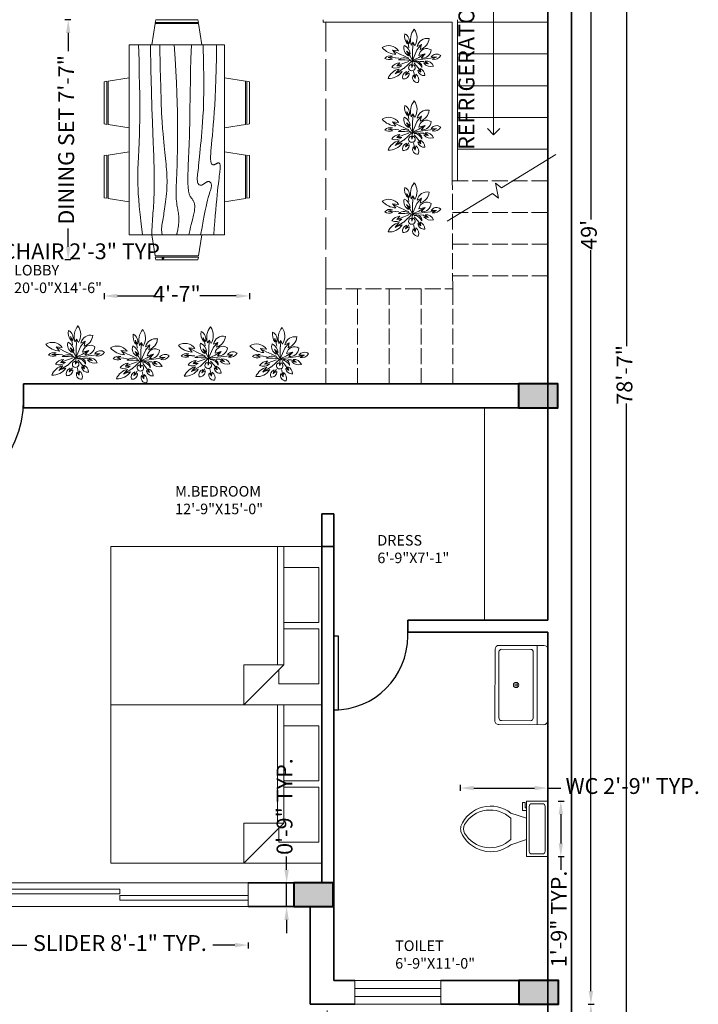
# Model space of a CAD drawing. Units: inches. Extents: x 2845 to 3575, y 808 to 1996.
# Tile 4 of 6: x 3304 to 3561, y 1215 to 1588. Entities that reach past the tile are written whole.
import ezdxf

# ---------------------------------------------------------------- set-up
doc = ezdxf.new("R2010")
doc.units = ezdxf.units.IN
doc.linetypes.add('ACAD_ISO02W100', pattern=[15, 12, -3])
for name, color, linetype, lineweight in [('A-ANNO-DIMS', 2, 'Continuous', 18), ('A-ANNO-SYMB', 7, 'Continuous', 18), ('A-AREA-IDEN', 7, 'Continuous', 18), ('A-COLS', 7, 'Continuous', 40), ('A-DOOR', 34, 'Continuous', 25), ('A-FLOR-CASE', 30, 'Continuous', 18), ('A-FLOR-FIXT', 8, 'Continuous', 18), ('A-FLOR-STRS', 142, 'Continuous', 18), ('A-FLOR-STRS-OVHD', 142, 'ACAD_ISO02W100', 18), ('A-FURN', 30, 'Continuous', 18), ('A-GLAZ', 4, 'Continuous', 18), ('A-ROOF-OVHD', 7, 'ACAD_ISO02W100', 18), ('A-WALL', 1, 'Continuous', 35), ('L-PLNT', 3, 'Continuous', 13)]:
    doc.layers.add(name, color=color, linetype=linetype, lineweight=lineweight)
doc.styles.get("Standard").update_dxf_attribs({"font": 'arial.ttf'})
doc.dimstyles.new('ISO-25', dxfattribs={"dimtxt": 6, "dimasz": 5, "dimexe": 1.25, "dimexo": 0.625, "dimtad": 0, "dimlunit": 4, "dimtxsty": 'Standard', "dimcen": 2.5, "dimclrd": 1, "dimclre": 1, "dimclrt": 1, "dimadec": 0, "dimazin": 0, "dimtfac": 1, "dimtmove": 0, "dimatfit": 3, "dimfxl": 1, "dimfxlon": 1, "dimfrac": 1, "dimarcsym": 0})

# ---------------------------------------------------------------- blocks, each defined once
blk = doc.blocks.new('*U5')
for p, q in [((0, 0), (0, 6)), ((40, 0), (40, 6))]:
    blk.add_line(p, q)
blk.add_lwpolyline([(0, 0), (0, -40), (1.75, -40), (1.75, 0)], close=True)
blk.add_arc((0, 0), 40, 270, 0)
blk = doc.blocks.new('*U6')
for p, q in [((0, 0), (0, 6)), ((28, 0), (28, 6))]:
    blk.add_line(p, q)
blk.add_lwpolyline([(0, 0), (0, -28), (1.75, -28), (1.75, 0)], close=True)
blk.add_arc((0, 0), 28, 270, 0)
blk = doc.blocks.new('Bed - Queen')
for p, q in [((0, -80.00003), (0, 0)), ((0, 0), (59.99999, 0)), ((59.99999, 0), (59.99999, -80.00003)), ((7.99999, -1.2), (28.79998, -1.2)), ((7.99999, -14.4), (7.99999, -1.2)), ((28.79998, -1.2), (28.79998, -14.4)), ((31.19999, -1.2), (51.99999, -1.2)), ((31.19999, -14.4), (31.19999, -1.2)), ((51.99999, -1.2), (51.99999, -16.4)), ((0, -14.4), (44.8, -14.4)), ((59.99999, -29.6), (44.8, -14.4)), ((44.8, -14.4), (44.8, -29.6)), ((44.8, -16.8), (0, -16.8)), ((51.99999, -16.4), (46.79936, -16.4)), ((44.8, -29.6), (59.99999, -29.6)), ((59.99999, -80.00003), (0, -80.00003))]:
    blk.add_line(p, q)
blk = doc.blocks.new('Dining Set - 36 x 72 in.')
for p, q in [((-22, 27.5), (-22.1562, 26.50042)), ((-5.8416, 26.5), (-22.1534, 26.5)), ((-22, 27.5), (-6, 27.5)), ((-5.8437, 26.49966), (-6, 27.5)), ((6, 27.5), (5.8438, 26.50042)), ((22.1584, 26.5), (5.8466, 26.5)), ((6, 27.5), (22, 27.5)), ((22.1563, 26.49966), (22, 27.5)), ((-22.2343, 26.00059), (-23.4847, 17.99762)), ((-22.2304, 26), (-5.7608, 26)), ((-4.5152, 17.99762), (-5.7655, 25.99926)), ((5.7657, 26.00059), (4.5153, 17.99762)), ((5.7696, 26), (22.2392, 26)), ((23.4848, 17.99762), (22.2345, 25.99926)), ((36, 18), (-36, 18)), ((-36, 18), (-36, -18)), ((36, -18), (36, 18)), ((-45.5, 8), (-44.5004, 8.15617)), ((-45.5, 8), (-45.5, -8)), ((-44.5, -8.15843), (-44.5, 8.15338)), ((-44.0006, 8.23428), (-35.9976, 9.48474)), ((-44, 8.23041), (-44, -8.23915)), ((44.0006, 8.23428), (35.9976, 9.48474)), ((44, 8.23041), (44, -8.23915)), ((44.5, -8.15843), (44.5, 8.15338)), ((45.5, 8), (44.5005, 8.15617)), ((45.5, 8), (45.5, -8)), ((-44.4997, -8.15631), (-45.5, -8)), ((-35.9976, -9.48476), (-43.9993, -8.2345)), ((35.9976, -9.48476), (43.9993, -8.2345)), ((44.4997, -8.15631), (45.5, -8)), ((-36, -18), (36, -18)), ((-22.2343, -26.0006), (-23.4847, -17.99762)), ((-4.5152, -17.99762), (-5.7655, -25.99928)), ((5.7657, -26.0006), (4.5153, -17.99762)), ((23.4848, -17.99762), (22.2345, -25.99928)), ((-22.2304, -26), (-5.7608, -26)), ((5.7696, -26), (22.2392, -26)), ((-22, -27.5), (-22.1562, -26.50044)), ((-5.8416, -26.5), (-22.1534, -26.5)), ((-22, -27.5), (-6, -27.5)), ((-5.8437, -26.49967), (-6, -27.5)), ((6, -27.5), (5.8438, -26.50044)), ((22.1584, -26.5), (5.8466, -26.5)), ((6, -27.5), (22, -27.5)), ((22.1563, -26.49967), (22, -27.5))]:
    blk.add_line(p, q)
for points in [[(-36, 15), (-31.1772, 14.97754), (-26.8079, 14.91406), (-22.8538, 14.81543), (-19.276, 14.6875), (-16.0362, 14.53613), (-13.0957, 14.36718), (-10.4159, 14.18652), (-7.9583, 14), (-5.6904, 13.81315), (-3.6035, 13.63021), (-1.6954, 13.45508), (0.0365, 13.29166), (1.5945, 13.14388), (2.9811, 13.01562), (4.1988, 12.9108), (5.25, 12.83333), (6.1393, 12.78613), (6.8802, 12.76823), (7.4883, 12.77767), (7.9792, 12.8125), (8.3685, 12.87077), (8.6719, 12.95052), (8.9049, 13.0498), (9.0833, 13.16666), (9.2205, 13.29899), (9.3216, 13.44401), (9.3895, 13.59879), (9.4271, 13.76041), (9.4373, 13.92594), (9.4232, 14.09245), (9.3875, 14.257), (9.3333, 14.41666), (9.2638, 14.56917), (9.1836, 14.71484), (9.0975, 14.85465), (9.0104, 14.98958), (8.9272, 15.1206), (8.8529, 15.2487), (8.7922, 15.37483), (8.75, 15.5), (8.7305, 15.62467), (8.7344, 15.74739), (8.7617, 15.86621), (8.8125, 15.97916), (8.8867, 16.08431), (8.9844, 16.17968), (9.1055, 16.26334), (9.25, 16.33333), (9.4189, 16.38802), (9.6172, 16.42708), (9.8506, 16.45052), (10.125, 16.45833), (10.4463, 16.45052), (10.8203, 16.42708), (11.2529, 16.38802), (11.75, 16.33333), (12.3184, 16.26318), (12.9694, 16.17838), (13.7151, 16.07991), (14.5677, 15.96875), (15.5395, 15.84586), (16.6426, 15.71224), (17.8893, 15.56884), (19.2917, 15.41666), (20.859, 15.25667), (22.5879, 15.08984), (24.4721, 14.91715), (26.5052, 14.73958), (28.6809, 14.5581), (30.9929, 14.3737), (33.4347, 14.18733), (36, 14)], [(-36, 10), (-28.9766, 10.14274), (-23.1725, 10.20442), (-18.4241, 10.19775), (-14.5677, 10.13541), (-11.4399, 10.03011), (-8.877, 9.89453), (-6.7154, 9.74137), (-4.7917, 9.58333), (-2.9698, 9.43082), (-1.2246, 9.28515), (0.4415, 9.14534), (2.026, 9.01041), (3.5266, 8.87939), (4.9408, 8.7513), (6.266, 8.62516), (7.5, 8.5), (8.6411, 8.37549), (9.6914, 8.2539), (10.6538, 8.13818), (11.5312, 8.03125), (12.3267, 7.93603), (13.043, 7.85547), (13.6831, 7.79248), (14.25, 7.75), (14.7471, 7.7303), (15.1797, 7.73307), (15.5537, 7.75732), (15.875, 7.80208), (16.1494, 7.86637), (16.3828, 7.94922), (16.5811, 8.04964), (16.75, 8.16666), (16.8944, 8.29915), (17.0143, 8.44531), (17.1089, 8.60319), (17.1771, 8.77083), (17.218, 8.94629), (17.2305, 9.1276), (17.2137, 9.31282), (17.1667, 9.5), (17.0895, 9.6875), (16.987, 9.875), (16.8649, 10.0625), (16.7292, 10.25), (16.5856, 10.4375), (16.4401, 10.625), (16.2985, 10.8125), (16.1667, 11), (16.05, 11.18733), (15.9518, 11.3737), (15.8752, 11.5581), (15.8229, 11.73958), (15.798, 11.91715), (15.8034, 12.08984), (15.842, 12.25667), (15.9167, 12.41666), (16.0295, 12.56836), (16.1784, 12.70833), (16.3605, 12.83268), (16.5729, 12.9375), (16.8127, 13.01888), (17.0768, 13.07291), (17.3625, 13.0957), (17.6667, 13.08333), (17.9894, 13.03312), (18.3418, 12.94726), (18.7382, 12.82918), (19.1927, 12.68229), (19.7195, 12.51001), (20.3327, 12.31575), (21.0465, 12.10294), (21.875, 11.875), (22.8357, 11.63354), (23.959, 11.37304), (25.2786, 11.08618), (26.8282, 10.76562), (28.6414, 10.40405), (30.752, 9.99414), (33.1936, 9.52856), (36, 9)], [(-36, 5.5), (-30.7157, 5.3348), (-26.069, 5.20963), (-21.9946, 5.11767), (-18.4271, 5.05208), (-15.3009, 5.00602), (-12.5508, 4.97265), (-10.1112, 4.94515), (-7.9167, 4.91666), (-5.909, 4.88167), (-4.0586, 4.83984), (-2.3429, 4.79215), (-0.7396, 4.73958), (0.7739, 4.6831), (2.22, 4.6237), (3.6213, 4.56233), (5, 4.5), (6.373, 4.43782), (7.7344, 4.3776), (9.0723, 4.32129), (10.375, 4.27083), (11.6309, 4.22819), (12.8281, 4.19531), (13.9551, 4.17415), (15, 4.16666), (15.954, 4.17448), (16.819, 4.19791), (17.6001, 4.23698), (18.3021, 4.29166), (18.9299, 4.36198), (19.4883, 4.44791), (19.9823, 4.54948), (20.4167, 4.66666), (20.7969, 4.79899), (21.1302, 4.94401), (21.4245, 5.09879), (21.6875, 5.26041), (21.9271, 5.42594), (22.1511, 5.59245), (22.3672, 5.757), (22.5834, 5.91666), (22.8065, 6.06868), (23.0404, 6.21093), (23.2879, 6.34147), (23.5521, 6.45833), (23.8358, 6.55957), (24.142, 6.64323), (24.4735, 6.70735), (24.8334, 6.75), (25.2235, 6.76969), (25.642, 6.76692), (26.0858, 6.74267), (26.5521, 6.69791), (27.0379, 6.63362), (27.5404, 6.55078), (28.0565, 6.45036), (28.5834, 6.33333), (29.1242, 6.19987), (29.7071, 6.04687), (30.3661, 5.87044), (31.1354, 5.66666), (32.0493, 5.43164), (33.142, 5.16146), (34.4475, 4.85221), (36, 4.5)], [(-36, -1), (-30.7915, -0.6591), (-26.0195, -0.38216), (-21.6519, -0.16284), (-17.6563, 0.00521), (-14.0005, 0.12833), (-10.6523, 0.21289), (-7.5796, 0.26522), (-4.75, 0.29166), (-2.134, 0.29793), (0.2878, 0.28711), (2.5317, 0.26163), (4.6146, 0.22396), (6.5529, 0.17651), (8.3633, 0.12174), (10.0623, 0.06209), (11.6667, 0), (13.1899, -0.06201), (14.6341, -0.1211), (15.9982, -0.17432), (17.2813, -0.21875), (18.4823, -0.25147), (19.6003, -0.26953), (20.6343, -0.27002), (21.5834, -0.25), (22.4481, -0.20768), (23.2357, -0.14584), (23.9549, -0.06836), (24.6146, 0.02083), (25.2235, 0.11784), (25.7904, 0.21875), (26.3241, 0.31966), (26.8334, 0.41666), (27.3265, 0.50618), (27.8099, 0.58593), (28.2894, 0.65397), (28.7709, 0.70833), (29.2601, 0.74707), (29.763, 0.76823), (30.2855, 0.76985), (30.8334, 0.75), (31.4088, 0.70784), (31.9994, 0.64713), (32.589, 0.57275), (33.1615, 0.48958), (33.7008, 0.4025), (34.1908, 0.3164), (34.6153, 0.23616), (34.9584, 0.16666), (35.2099, 0.11165), (35.3848, 0.07031), (35.504, 0.04069), (35.5886, 0.02083), (35.6594, 0.00879), (35.7377, 0.0026), (35.8442, 0.00032), (36, 0)], [(-36, -6.5), (-27.1843, -6.31267), (-20.084, -6.1263), (-14.469, -5.9419), (-10.1094, -5.76042), (-6.7752, -5.58285), (-4.2363, -5.41016), (-2.2629, -5.24333), (-0.625, -5.08334), (0.8708, -4.93099), (2.2715, -4.78646), (3.5872, -4.64974), (4.8281, -4.52084), (6.0046, -4.39974), (7.127, -4.28646), (8.2053, -4.18099), (9.25, -4.08334), (10.2705, -3.99382), (11.2734, -3.91407), (12.2647, -3.84603), (13.25, -3.79167), (14.2354, -3.75293), (15.2266, -3.73177), (16.2295, -3.73015), (17.25, -3.75), (18.2912, -3.79248), (19.3451, -3.85547), (20.4009, -3.93604), (21.4479, -4.03125), (22.4754, -4.13819), (23.4727, -4.25391), (24.4289, -4.37549), (25.3334, -4.5), (26.1785, -4.62492), (26.9694, -4.74935), (27.7145, -4.87281), (28.4219, -4.99479), (29.1, -5.11483), (29.7572, -5.23242), (30.4016, -5.34709), (31.0417, -5.45834), (31.6837, -5.56437), (32.3262, -5.65821), (32.9658, -5.73153), (33.599, -5.77604), (34.2224, -5.78345), (34.8327, -5.74545), (35.4264, -5.65373), (36, -5.5)], [(-36, -10), (-26.4022, -9.81299), (-18.4675, -9.62891), (-11.9839, -9.45069), (-6.7396, -9.28125), (-2.5226, -9.12354), (0.8789, -8.98047), (3.6769, -8.85498), (6.0833, -8.75), (8.2767, -8.66765), (10.3021, -8.60677), (12.1712, -8.56543), (13.8958, -8.54167), (15.4876, -8.53353), (16.9583, -8.53907), (18.3197, -8.55632), (19.5834, -8.58334), (20.7616, -8.61841), (21.8685, -8.66081), (22.9188, -8.71004), (23.9271, -8.76563), (24.9081, -8.82707), (25.8763, -8.89388), (26.8465, -8.96558), (27.8334, -9.04167), (28.8474, -9.12118), (29.8828, -9.20117), (30.93, -9.27824), (31.9792, -9.34896), (33.0205, -9.40991), (34.0443, -9.45768), (35.0407, -9.48885), (36, -9.5)], [(-36, -14.5), (-30.0881, -14.33513), (-25.0332, -14.21224), (-20.7312, -14.12647), (-17.0781, -14.07292), (-13.97, -14.04671), (-11.3027, -14.04297), (-8.9724, -14.05681), (-6.875, -14.08334), (-4.9224, -14.11833), (-3.0905, -14.16016), (-1.3709, -14.20785), (0.2448, -14.26042), (1.7647, -14.3169), (3.1973, -14.3763), (4.5507, -14.43767), (5.8333, -14.5), (7.0554, -14.5621), (8.235, -14.62175), (9.3922, -14.67652), (10.5469, -14.72396), (11.7192, -14.76164), (12.929, -14.78711), (14.1965, -14.79794), (15.5417, -14.79167), (16.9933, -14.76424), (18.6152, -14.70508), (20.4804, -14.60197), (22.6615, -14.44271), (25.2312, -14.21509), (28.2624, -13.9069), (31.8277, -13.50594), (36, -13)]]:
    blk.add_lwpolyline(points)
blk = doc.blocks.new('Sink-single - 30 in top')
blk.add_line((-15, -3.999996), (15, -3.999996))
for points in [[(-13.5, 0), (13.5, 0)], [(-15, -18.499996), (-15, -1.5)], [(15, -1.5), (15, -18.499996)], [(-13.5, -17.499996), (-13.5, -6.499996)], [(-12.5, -5.499996), (12.5, -5.499996)], [(13.5, -6.499996), (13.5, -17.499996)], [(12.5, -18.499996), (-12.5, -18.499996)], [(13.5, -19.999996), (-13.5, -19.999996)]]:
    blk.add_lwpolyline(points)
for radius in [1, 0.5]:
    blk.add_circle((0, -11.999996), radius)
for centre, radius, start, end in [((-13.5, -1.5), 1.5, 90, 180), ((13.5, -1.5), 1.5, 0, 90), ((-12.5, -6.499996), 1, 90, 180), ((12.5, -6.499996), 1, 0, 90), ((-13.5, -18.499996), 1.5, 180, 270), ((-12.5, -17.499996), 1, 180, 270), ((12.5, -17.499996), 1, 270, 0), ((13.5, -18.499996), 1.5, 270, 0)]:
    blk.add_arc(centre, radius, start, end)
blk = doc.blocks.new('Toilet - top')
for p, q in [((9.5, -6), (9.5, -2)), ((-10, -8.5), (-8, -8.5)), ((-10, -9.5), (-10, -8.5)), ((-7, -9.5), (-10, -9.5)), ((-8, -8.5), (-8, -8)), ((-7, -8), (-7, -9.5)), ((-4, -8), (-6, -14)), ((4, -8), (6, -14)), ((4, -14), (-4, -14))]:
    blk.add_line(p, q)
blk.add_lwpolyline([(10.5, -8), (10.5, 0), (-10.5, 0), (-10.5, -8)], close=True)
for points in [[(-9.5, -2), (-9.5, -6)], [(8.5, -1), (-8.5, -1)], [(-8.5, -7), (8.5, -7)]]:
    blk.add_lwpolyline(points)
for centre, radius, start, end in [((-8.62, -1.88), 0.884, 81.8699, 188.1301), ((8.62, -1.88), 0.884, 351.8699, 98.1301), ((-8.62, -6.12), 0.884, 171.8699, 278.1301), ((8.62, -6.12), 0.884, 261.8699, 8.1301), ((3.52, -21.58), 12.17, 141.4691, 247.9714), ((4.2, -21.82), 11.33, 136.3677, 238.9468), ((-3.52, -21.58), 12.17, 292.0284, 38.5307), ((-4.2, -21.82), 11.33, 301.053, 43.6321), ((0, -27.88), 4, 245.7318, 294.2682), ((0, -29), 4, 254.8605, 285.1395)]:
    blk.add_arc(centre, radius, start, end)
blk = doc.blocks.new('z_109')
for p, q in [((-94, 294), (-122, 396)), ((-121, 393), (-119, 324)), ((-120, 377), (-82, 322)), ((-392, 202), (-278, 190)), ((-254, 128), (-392, 202)), ((-390, 202), (-327, 125)), ((-61, 92), (-128, 186)), ((-85, 244), (-94, 293)), ((-5, 350), (-42, 295)), ((-20, 11), (-18, 230)), ((-20, 11), (65, 205)), ((-14, 234), (-5, 350)), ((-5, 350), (24, 284)), ((65, 209), (150, 307)), ((65, 205), (65, 205)), ((150, 307), (68, 272)), ((129, 216), (150, 307)), ((150, 307), (129, 216)), ((-342, 60), (-472, 63)), ((-467, 63), (-392, 90)), ((-463, 64), (-392, 37)), ((-276, 53), (-338, 57)), ((-84, 54), (-246, 125)), ((-20, 11), (-181, -143)), ((-126, 184), (-60, 125)), ((-120, 176), (-91, 98)), ((-20, 11), (-61, 92)), ((-20, 11), (-24, -65)), ((-20, 11), (102, 64)), ((-20, 11), (-14, 11)), ((-14, 11), (319, 50)), ((-14, 11), (-13, 13)), ((-13, 13), (13, -13)), ((217, 135), (101, 105)), ((102, 64), (217, 135)), ((217, 135), (145, 55)), ((319, 50), (434, 75)), ((429, 74), (333, 77)), ((428, 74), (353, 32)), ((-187, -143), (-345, -240)), ((-342, -238), (-269, -151)), ((-178, -41), (-313, -92)), ((-308, -90), (-254, -33)), ((-306, -89), (-217, -88)), ((-86, -8), (-178, -41)), ((-26, -113), (-45, -66)), ((-24, -65), (-28, -121)), ((-28, -117), (-2, -69)), ((16, -43), (88, -126)), ((141, -208), (84, -170)), ((87, -129), (140, -204)), ((122, -8), (193, -11)), ((140, -205), (123, -139)), ((176, -10), (285, -54)), ((283, -54), (196, -42)), ((273, -52), (222, -4)), ((-328, -230), (-213, -195)), ((-151, -267), (-81, -228)), ((-89, -192), (-150, -267)), ((-150, -266), (-131, -199)), ((34, -320), (-6, -268)), ((4, -192), (16, -238)), ((16, -238), (35, -326)), ((35, -327), (45, -249))]:
    blk.add_line(p, q)
for centre, radius, start, end in [((262, 393), 319, 140.563, 197.8988), ((-221, 433), 288, 328.6458, 34.5329), ((84, 468), 249, 170.3029, 215.3262), ((-235, 368), 160, 343.2534, 62.5239), ((256, 231), 192, 77.7318, 167.6805), ((55, 447), 242, 287.7269, 353.3689), ((-464, 59), 228, 35.1725, 122.5976), ((-304, 504), 380, 221.8384, 266.6027), ((-21, 239), 158, 161.4501, 243.415), ((-251, 115), 192, 2.9136, 65.0019), ((247, 86), 147, 55.2824, 172.6291), ((167, 217), 164, 262.2896, 356.2544), ((-434, -39), 136, 71.6414, 139.5892), ((-450, 225), 197, 243.5199, 287.2599), ((-173, -118), 175, 44.3837, 127.1057), ((-243, -1063), 1086, 79.6239, 91.8656), ((434, 8), 123, 51.1111, 145.9654), ((384, 175), 146, 257.8549, 330.7421), ((-198, -444), 302, 103.499, 156.8265), ((-246, -222), 190, 92.4489, 147.0817), ((-337, 52), 185, 248.0932, 310.529), ((-31, -123), 58.9, 103.4106, 268.148), ((-26, -123), 58.9, 262.5922, 66.6581), ((53, -110), 105, 354.7987, 111.9005), ((2, -181), 167, 21.6922, 85.2277), ((197, -160), 113, 185.1842, 278.9266), ((66, -276), 148, 1.4924, 67.3596), ((325, 60), 164, 218.6232, 288.4099), ((241, -149), 146, 21.4559, 97.3107), ((-455, -39), 287, 265.8156, 327.2626), ((-94, -301), 109, 109.8936, 199.3062), ((-186, -232), 105, 264.4232, 2.0221), ((80, -308), 95.1, 155.1092, 275.9038), ((-28, -354), 128, 337.3115, 55.0978)]:
    blk.add_arc(centre, radius, start, end)
blk = doc.blocks.new('*D27')
at = {"layer": 'A-ANNO-DIMS', "color": 0, "lineweight": -2, "transparency": 16777216}
for p, q in [((3518.95, 1798.17), (3521.2, 1798.17)), ((3519.95, 1793.17), (3519.95, 1512.51)), ((3519.95, 1220.17), (3519.95, 1500.84)), ((3518.95, 1215.17), (3521.2, 1215.17))]:
    blk.add_line(p, q, dxfattribs=at)
at = {"layer": 'A-ANNO-DIMS', "color": 0, "transparency": 16777216}
for points in [[(3519.11, 1793.17), (3520.78, 1793.17), (3519.95, 1798.17)], [(3519.11, 1220.17), (3520.78, 1220.17), (3519.95, 1215.17)]]:
    blk.add_solid(points, dxfattribs=at)
at = {"layer": 'Defpoints', "color": 0, "transparency": 16777216}
for p in [(3512.62, 1798.17), (3507.65, 1215.17), (3519.95, 1215.17)]:
    blk.add_point(p, dxfattribs=at)
at = {"layer": 'A-ANNO-DIMS', "color": 0, "transparency": 16777216, "insert": (3519.95, 1506.67), "char_height": 6, "attachment_point": 5, "rotation": 90}
blk.add_mtext("49'", dxfattribs=at)
blk = doc.blocks.new('*D28')
at = {"layer": 'A-ANNO-DIMS', "color": 0, "lineweight": -2, "transparency": 16777216}
for p, q in [((3518.95, 1215.17), (3521.2, 1215.17)), ((3519.95, 1210.17), (3519.95, 1104.11)), ((3519.95, 987.17), (3519.95, 1093.24)), ((3518.95, 982.17), (3521.2, 982.17))]:
    blk.add_line(p, q, dxfattribs=at)
at = {"layer": 'A-ANNO-DIMS', "color": 0, "transparency": 16777216}
for points in [[(3519.11, 1210.17), (3520.78, 1210.17), (3519.95, 1215.17)], [(3519.11, 987.17), (3520.78, 987.17), (3519.95, 982.17)]]:
    blk.add_solid(points, dxfattribs=at)
at = {"layer": 'Defpoints', "color": 0, "transparency": 16777216}
for p in [(3507.65, 1215.17), (3512.62, 982.17), (3519.95, 982.17)]:
    blk.add_point(p, dxfattribs=at)
at = {"layer": 'A-ANNO-DIMS', "color": 0, "transparency": 16777216, "insert": (3519.95, 1098.67), "char_height": 6, "attachment_point": 5, "rotation": 90}
blk.add_mtext("19'", dxfattribs=at)
blk = doc.blocks.new('*D29')
at = {"layer": 'A-ANNO-DIMS', "color": 0, "lineweight": -2, "transparency": 16777216}
for p, q in [((3532.44, 1925.07), (3534.69, 1925.07)), ((3533.44, 1920.07), (3533.44, 1464.53)), ((3533.44, 987.17), (3533.44, 1442.72)), ((3532.44, 982.17), (3534.69, 982.17))]:
    blk.add_line(p, q, dxfattribs=at)
at = {"layer": 'A-ANNO-DIMS', "color": 0, "transparency": 16777216}
for points in [[(3532.6, 1920.07), (3534.27, 1920.07), (3533.44, 1925.07)], [(3532.6, 987.17), (3534.27, 987.17), (3533.44, 982.17)]]:
    blk.add_solid(points, dxfattribs=at)
at = {"layer": 'Defpoints', "color": 0, "transparency": 16777216}
for p in [(3519.95, 1925.07), (3533.44, 1925.07), (3512.62, 982.17)]:
    blk.add_point(p, dxfattribs=at)
at = {"layer": 'A-ANNO-DIMS', "color": 0, "transparency": 16777216, "insert": (3533.44, 1453.62), "char_height": 6, "attachment_point": 5, "rotation": 90}
blk.add_mtext('78\'-7"', dxfattribs=at)
blk = doc.blocks.new('COL-15x9')
h = blk.add_hatch(color=256)
h.dxf.hatch_style = 1
h.paths.add_polyline_path([(15, 9), (0, 9), (0, 0), (15, 0)])
blk.add_lwpolyline([(0, 9), (0, 0), (15, 0), (15, 9)], close=True)
blk = doc.blocks.new('GLAZ-SLIDER-97')
for p, q in [((0, 9), (0, 0)), ((0, 9), (97.12, 9)), ((97.12, 9), (97.12, 0)), ((0, 6.63), (48.56, 6.63)), ((48.56, 4.89), (0, 4.89)), ((48.56, 6.63), (48.56, 4.89)), ((48.56, 2.45), (48.56, 4.19)), ((48.56, 4.19), (97.12, 4.19)), ((0, 0), (97.12, 0)), ((97.12, 2.45), (48.56, 2.45))]:
    blk.add_line(p, q)
blk = doc.blocks.new('*D56')
at = {"layer": 'A-ANNO-DIMS', "color": 1, "lineweight": -2, "transparency": 16777216}
for p, q in [((3262.84, 1500.65), (3262.84, 1498.4)), ((3267.84, 1499.65), (3284.84, 1499.65)), ((3289.84, 1500.65), (3289.84, 1498.4)), ((3289.84, 1499.65), (3294.84, 1499.65))]:
    blk.add_line(p, q, dxfattribs=at)
at = {"layer": 'A-ANNO-DIMS', "color": 1, "transparency": 16777216}
for points in [[(3267.84, 1500.49), (3267.84, 1498.82), (3262.84, 1499.65)], [(3284.84, 1500.49), (3284.84, 1498.82), (3289.84, 1499.65)]]:
    blk.add_solid(points, dxfattribs=at)
at = {"layer": 'Defpoints', "color": 0, "transparency": 16777216}
for p in [(3262.84, 1503.7), (3289.84, 1503.7), (3289.84, 1499.65)]:
    blk.add_point(p, dxfattribs=at)
at = {"layer": 'A-ANNO-DIMS', "color": 1, "transparency": 16777216, "insert": (3327.92, 1499.65), "char_height": 6, "attachment_point": 5}
blk.add_mtext('CHAIR 2\'-3" TYP.', dxfattribs=at)
blk = doc.blocks.new('*D62')
at = {"layer": 'A-ANNO-DIMS', "color": 1, "lineweight": -2, "transparency": 16777216}
for p, q in [((3470.57, 1296.09), (3470.57, 1298.34)), ((3503.62, 1296.09), (3503.62, 1298.34)), ((3475.57, 1297.09), (3498.62, 1297.09)), ((3503.62, 1297.09), (3508.62, 1297.09))]:
    blk.add_line(p, q, dxfattribs=at)
at = {"layer": 'A-ANNO-DIMS', "color": 1, "transparency": 16777216}
for points in [[(3475.57, 1297.93), (3475.57, 1296.26), (3470.57, 1297.09)], [(3498.62, 1297.93), (3498.62, 1296.26), (3503.62, 1297.09)]]:
    blk.add_solid(points, dxfattribs=at)
at = {"layer": 'Defpoints', "color": 0, "transparency": 16777216}
for p in [(3503.62, 1297.09), (3470.57, 1292.14), (3503.62, 1292.14)]:
    blk.add_point(p, dxfattribs=at)
at = {"layer": 'A-ANNO-DIMS', "color": 1, "transparency": 16777216, "insert": (3535.8, 1297.09), "char_height": 6, "attachment_point": 5}
blk.add_mtext('WC 2\'-9" TYP.', dxfattribs=at)
blk = doc.blocks.new('*D63')
at = {"layer": 'A-ANNO-DIMS', "color": 1, "lineweight": -2, "transparency": 16777216}
for p, q in [((3507.57, 1292.14), (3509.82, 1292.14)), ((3508.57, 1287.14), (3508.57, 1276.14)), ((3507.57, 1271.14), (3509.82, 1271.14)), ((3508.57, 1271.14), (3508.57, 1266.14))]:
    blk.add_line(p, q, dxfattribs=at)
at = {"layer": 'A-ANNO-DIMS', "color": 1, "transparency": 16777216}
for points in [[(3507.74, 1287.14), (3509.41, 1287.14), (3508.57, 1292.14)], [(3507.74, 1276.14), (3509.41, 1276.14), (3508.57, 1271.14)]]:
    blk.add_solid(points, dxfattribs=at)
at = {"layer": 'Defpoints', "color": 0, "transparency": 16777216}
for p in [(3503.62, 1292.14), (3503.62, 1271.14), (3508.57, 1271.14)]:
    blk.add_point(p, dxfattribs=at)
at = {"layer": 'A-ANNO-DIMS', "color": 1, "transparency": 16777216, "insert": (3508.57, 1247.51), "char_height": 6, "attachment_point": 5, "rotation": 90}
blk.add_mtext('1\'-9" TYP.', dxfattribs=at)
blk = doc.blocks.new('*D64')
at = {"layer": 'A-ANNO-DIMS', "color": 1, "lineweight": -2, "transparency": 16777216}
for p, q in [((3293.03, 1238.6), (3293.03, 1236.35)), ((3390.15, 1238.6), (3390.15, 1236.35)), ((3298.03, 1237.6), (3306.39, 1237.6)), ((3385.15, 1237.6), (3376.79, 1237.6))]:
    blk.add_line(p, q, dxfattribs=at)
at = {"layer": 'A-ANNO-DIMS', "color": 1, "transparency": 16777216}
for points in [[(3298.03, 1238.44), (3298.03, 1236.77), (3293.03, 1237.6)], [(3385.15, 1238.44), (3385.15, 1236.77), (3390.15, 1237.6)]]:
    blk.add_solid(points, dxfattribs=at)
at = {"layer": 'Defpoints', "color": 0, "transparency": 16777216}
for p in [(3293.03, 1252.17), (3390.15, 1252.17), (3390.15, 1237.6)]:
    blk.add_point(p, dxfattribs=at)
at = {"layer": 'A-ANNO-DIMS', "color": 1, "transparency": 16777216, "insert": (3341.59, 1237.6), "char_height": 6, "attachment_point": 5}
blk.add_mtext('SLIDER 8\'-1" TYP.', dxfattribs=at)
blk = doc.blocks.new('*D65')
at = {"layer": 'A-ANNO-DIMS', "color": 1, "lineweight": -2, "transparency": 16777216}
for p, q in [((3404.72, 1266.17), (3404.72, 1271.17)), ((3403.72, 1261.17), (3405.97, 1261.17)), ((3404.72, 1252.17), (3404.72, 1261.17)), ((3403.72, 1252.17), (3405.97, 1252.17)), ((3404.72, 1247.17), (3404.72, 1242.17))]:
    blk.add_line(p, q, dxfattribs=at)
at = {"layer": 'A-ANNO-DIMS', "color": 1, "transparency": 16777216}
for points in [[(3403.89, 1266.17), (3405.55, 1266.17), (3404.72, 1261.17)], [(3403.89, 1247.17), (3405.55, 1247.17), (3404.72, 1252.17)]]:
    blk.add_solid(points, dxfattribs=at)
at = {"layer": 'Defpoints', "color": 0, "transparency": 16777216}
for p in [(3390.15, 1261.17), (3404.72, 1261.17), (3390.15, 1252.17)]:
    blk.add_point(p, dxfattribs=at)
at = {"layer": 'A-ANNO-DIMS', "color": 1, "transparency": 16777216, "insert": (3404.72, 1290.08), "char_height": 6, "attachment_point": 5, "rotation": 90}
blk.add_mtext('0\'-9" TYP.', dxfattribs=at)
blk = doc.blocks.new('*D66')
at = {"layer": 'A-ANNO-DIMS', "color": 1, "lineweight": -2, "transparency": 16777216}
for p, q in [((3323.01, 1588.16), (3320.76, 1588.16)), ((3322.01, 1583.16), (3322.01, 1576.26)), ((3322.01, 1502.16), (3322.01, 1509.07)), ((3323.01, 1497.16), (3320.76, 1497.16))]:
    blk.add_line(p, q, dxfattribs=at)
at = {"layer": 'A-ANNO-DIMS', "color": 1, "transparency": 16777216}
for points in [[(3321.17, 1583.16), (3322.84, 1583.16), (3322.01, 1588.16)], [(3321.17, 1502.16), (3322.84, 1502.16), (3322.01, 1497.16)]]:
    blk.add_solid(points, dxfattribs=at)
at = {"layer": 'Defpoints', "color": 0, "transparency": 16777216}
for p in [(3335.66, 1588.16), (3322.01, 1497.16), (3335.66, 1497.16)]:
    blk.add_point(p, dxfattribs=at)
at = {"layer": 'A-ANNO-DIMS', "color": 1, "transparency": 16777216, "insert": (3322.01, 1542.66), "char_height": 6, "attachment_point": 5, "rotation": 90}
blk.add_mtext('DINING SET 7\'-7"', dxfattribs=at)
blk = doc.blocks.new('*D67')
at = {"layer": 'A-ANNO-DIMS', "color": 1, "lineweight": -2, "transparency": 16777216}
for p, q in [((3335.66, 1484.51), (3335.66, 1482.26)), ((3340.66, 1483.51), (3354.44, 1483.51)), ((3385.66, 1483.51), (3371.88, 1483.51)), ((3390.66, 1484.51), (3390.66, 1482.26))]:
    blk.add_line(p, q, dxfattribs=at)
at = {"layer": 'A-ANNO-DIMS', "color": 1, "transparency": 16777216}
for points in [[(3340.66, 1484.35), (3340.66, 1482.68), (3335.66, 1483.51)], [(3385.66, 1484.35), (3385.66, 1482.68), (3390.66, 1483.51)]]:
    blk.add_solid(points, dxfattribs=at)
at = {"layer": 'Defpoints', "color": 0, "transparency": 16777216}
for p in [(3335.66, 1497.16), (3390.66, 1497.16), (3390.66, 1483.51)]:
    blk.add_point(p, dxfattribs=at)
at = {"layer": 'A-ANNO-DIMS', "color": 1, "transparency": 16777216, "insert": (3363.16, 1483.51), "char_height": 6, "attachment_point": 5}
blk.add_mtext('4\'-7"', dxfattribs=at)
blk = doc.blocks.new('*D68')
at = {"layer": 'A-ANNO-DIMS', "color": 1, "lineweight": -2, "transparency": 16777216}
for p, q in [((3474.59, 1671.66), (3472.34, 1671.66)), ((3473.59, 1666.66), (3473.59, 1645.24)), ((3474.59, 1640.24), (3472.34, 1640.24)), ((3473.59, 1640.24), (3473.59, 1635.24))]:
    blk.add_line(p, q, dxfattribs=at)
at = {"layer": 'A-ANNO-DIMS', "color": 1, "transparency": 16777216}
for points in [[(3472.76, 1666.66), (3474.42, 1666.66), (3473.59, 1671.66)], [(3472.76, 1645.24), (3474.42, 1645.24), (3473.59, 1640.24)]]:
    blk.add_solid(points, dxfattribs=at)
at = {"layer": 'Defpoints', "color": 0, "transparency": 16777216}
for p in [(3478.3, 1671.66), (3473.59, 1640.24), (3478.3, 1640.24)]:
    blk.add_point(p, dxfattribs=at)
at = {"layer": 'A-ANNO-DIMS', "color": 1, "transparency": 16777216, "insert": (3473.59, 1585.34), "char_height": 6, "attachment_point": 5, "rotation": 90}
blk.add_mtext('REFRIGERATOR 2\'-7 1/2"', dxfattribs=at)

msp = doc.modelspace()

# ---------------------------------------------------------------- linework, layer by layer
at = {"layer": 'A-ANNO-SYMB'}
for p, q in [((3483.127, 1611.198), (3483.127, 1544.532)), ((3483.127, 1544.532), (3480.77, 1546.888)), ((3483.127, 1544.532), (3485.484, 1546.888))]:
    msp.add_line(p, q, dxfattribs=at)
at = {"layer": 'A-DOOR'}
for p, q in [((3305.116, 1450.173), (3305.116, 1441.173)), ((3450.616, 1360.673), (3450.616, 1356.173))]:
    msp.add_line(p, q, dxfattribs=at)
at = {"layer": 'A-FLOR-CASE'}
msp.add_line((3479.616, 1360.673), (3479.616, 1441.173), dxfattribs=at)
at = {"layer": 'A-FLOR-STRS'}
for p, q in [((3418.616, 1587.173), (3418.616, 1588.173)), ((3419.616, 1587.173), (3418.616, 1587.173)), ((3467.473, 1587.173), (3419.616, 1587.173)), ((3467.473, 1527.173), (3467.473, 1587.173)), ((3469.473, 1588.173), (3469.473, 1527.173)), ((3469.473, 1587.173), (3503.616, 1587.173)), ((3469.473, 1575.173), (3503.616, 1575.173)), ((3469.473, 1563.173), (3503.616, 1563.173)), ((3469.473, 1551.173), (3503.616, 1551.173)), ((3469.473, 1539.173), (3503.616, 1539.173)), ((3469.473, 1527.173), (3467.473, 1527.173))]:
    msp.add_line(p, q, dxfattribs=at)
msp.add_lwpolyline([(3465.584, 1511.835), (3482.73, 1522.371), (3485.02, 1520.554), (3483.847, 1526.283), (3486.138, 1524.465), (3506.721, 1537.114)], dxfattribs=at)
at = {"layer": 'A-FLOR-STRS-OVHD'}
msp.add_line((3419.616, 1486.173), (3419.616, 1587.173), dxfattribs=at)
at = {"layer": 'A-FLOR-STRS-OVHD', "ltscale": 0.5}
for p, q in [((3467.616, 1486.173), (3467.473, 1527.173)), ((3467.473, 1527.173), (3503.616, 1527.173)), ((3467.515, 1515.173), (3503.616, 1515.173)), ((3467.557, 1503.173), (3503.616, 1503.173)), ((3467.598, 1491.173), (3503.616, 1491.173)), ((3419.616, 1450.173), (3419.616, 1486.173)), ((3419.616, 1486.173), (3467.616, 1486.173)), ((3431.616, 1450.173), (3431.616, 1486.173)), ((3443.616, 1450.173), (3443.616, 1486.173)), ((3455.616, 1450.173), (3455.616, 1486.173)), ((3467.616, 1450.173), (3467.616, 1486.173))]:
    msp.add_line(p, q, dxfattribs=at)
at = {"layer": 'A-GLAZ'}
for p, q in [((3430.545, 1224.173), (3430.545, 1215.173)), ((3430.545, 1224.173), (3463.116, 1224.173)), ((3463.116, 1224.173), (3463.116, 1215.173)), ((3430.545, 1221.173), (3463.116, 1221.173)), ((3430.545, 1218.173), (3463.116, 1218.173)), ((3430.545, 1215.173), (3463.116, 1215.173))]:
    msp.add_line(p, q, dxfattribs=at)
at = {"layer": 'A-ROOF-OVHD'}
msp.add_line((3420.121, 1170.861), (3420.121, 1215.173), dxfattribs=at)
at = {"layer": 'A-WALL'}
for p, q in [((3512.616, 1159.066), (3512.616, 1798.173)), ((3503.616, 1450.173), (3503.616, 1624.173)), ((3503.616, 1450.173), (3305.116, 1450.173)), ((3503.616, 1441.173), (3503.616, 1450.173)), ((3503.616, 1441.173), (3305.116, 1441.173)), ((3503.616, 1360.673), (3503.616, 1441.173)), ((3418.116, 1261.173), (3418.116, 1400.934)), ((3418.116, 1400.934), (3422.616, 1400.934)), ((3422.616, 1252.173), (3422.616, 1400.934)), ((3418.116, 1388.635), (3422.616, 1388.635)), ((3503.616, 1360.673), (3450.616, 1360.673)), ((3503.616, 1356.173), (3450.616, 1356.173)), ((3503.616, 1159.066), (3503.616, 1356.173)), ((3422.616, 1261.173), (3390.151, 1261.173)), ((3422.616, 1224.173), (3422.616, 1261.173)), ((3422.616, 1252.173), (3390.151, 1252.173)), ((3413.616, 1215.173), (3413.616, 1252.173)), ((3503.616, 1224.173), (3503.616, 1252.173)), ((3430.545, 1224.173), (3422.616, 1224.173)), ((3503.616, 1224.173), (3463.116, 1224.173)), ((3422.616, 1215.173), (3413.616, 1215.173)), ((3430.545, 1215.173), (3422.616, 1215.173)), ((3503.616, 1215.173), (3463.116, 1215.173))]:
    msp.add_line(p, q, dxfattribs=at)

# ---------------------------------------------------------------- block references
at = {"layer": 'A-COLS'}
for p in [(3492.483, 1441.173), (3407.396, 1252.173), (3492.652, 1215.173)]:
    msp.add_blockref('COL-15x9', p, dxfattribs=at)
at = {"layer": 'A-DOOR'}
for name, p in [('*U5', (3265.116, 1444.173)), ('*U6', (3422.616, 1354.673))]:
    msp.add_blockref(name, p, dxfattribs=at)
at = {"layer": 'A-FLOR-FIXT'}
for name, p, rotation in [('Sink-single - 30 in top', (3503.616, 1336.103), 269.8478361324268), ('Toilet - top', (3503.616, 1281.637), 270)]:
    msp.add_blockref(name, p, dxfattribs=dict(at, rotation=rotation))
at = {"layer": 'A-FURN', "rotation": 270}
for name, p in [('Dining Set - 36 x 72 in.', (3363.156, 1542.665)), ('Bed - Queen', (3418.116, 1388.635)), ('Bed - Queen', (3418.116, 1328.635))]:
    msp.add_blockref(name, p, dxfattribs=at)
at = {"layer": 'A-GLAZ'}
msp.add_blockref('GLAZ-SLIDER-97', (3293.028, 1252.173), dxfattribs=at)
at = {"layer": 'L-PLNT', "xscale": 0.0202275909996564, "yscale": 0.0202275909996564, "zscale": 0.0202275909996564}
for p in [(3452.749, 1572.525), (3452.749, 1545.382), (3452.749, 1514.347), (3325.389, 1460.122), (3349.909, 1458.75), (3375.605, 1459.73), (3402.675, 1459.534)]:
    msp.add_blockref('z_109', p, dxfattribs=at)

# ---------------------------------------------------------------- texts
at = {"layer": 'A-AREA-IDEN', "char_height": 4, "attachment_point": 1}
for s, insert in [('LOBBY\\P20\'-0"X14\'-6"', (3301.502, 1495.272)), ('M.BEDROOM\\P12\'-9"X15\'-0"', (3362.52, 1411.503)), ('DRESS\\P6\'-9"X7\'-1"', (3439.088, 1392.956)), ('TOILET\\P6\'-9"X11\'-0"', (3445.829, 1239.356))]:
    msp.add_mtext_dynamic_manual_height_columns(s, width=45.255, gutter_width=12.5, heights=[0], dxfattribs=dict(at, insert=insert))

# ---------------------------------------------------------------- dimensions: what is measured, and where the dimension line sits
at = {"layer": 'A-ANNO-DIMS'}
dim = msp.add_linear_dim(base=(3533.438, 1925.073), p1=(3512.616, 982.173), p2=(3519.947, 1925.073), angle=90, dimstyle='ISO-25', override={"dimclrd": 0, "dimclre": 0, "dimclrt": 0}, dxfattribs=at)
dim.commit()
dim.dimension.update_dxf_attribs({"geometry": '*D29', "text_midpoint": (3533.438, 1453.623)})
for base, p1, p2, angle, text, override, picture, middle in [((3519.947, 1215.173), (3512.616, 1798.173), (3507.652, 1215.173), 90, "49'", {"dimclrd": 0, "dimclre": 0, "dimclrt": 0, "dimtmove": 1}, '*D27', (3519.947, 1506.673)), ((3473.59, 1640.236), (3478.303, 1671.658), (3478.303, 1640.236), 270, 'REFRIGERATOR <>', {"dimdec": 1, "dimlfac": 1, "dimrnd": 0, "dimzin": 1, "dimdsep": 46, "dimlunit": 4, "dimfrac": 2}, '*D68', (3473.59, 1585.34)), ((3322.006, 1497.165), (3335.656, 1588.165), (3335.656, 1497.165), 270, 'DINING SET <>', {"dimdec": 1, "dimlfac": 1, "dimrnd": 0, "dimzin": 1, "dimdsep": 46, "dimlunit": 4, "dimfrac": 2}, '*D66', (3322.006, 1542.665)), ((3404.72, 1261.173), (3390.151, 1252.173), (3390.151, 1261.173), 90, '<> TYP.', {"dimdec": 1, "dimlfac": 1, "dimrnd": 0, "dimzin": 1, "dimdsep": 46, "dimlunit": 4, "dimfrac": 2}, '*D65', (3404.72, 1290.084)), ((3508.573, 1271.137), (3503.616, 1292.137), (3503.616, 1271.137), 270, '<> TYP.', {"dimdec": 1, "dimlfac": 1, "dimrnd": 0, "dimzin": 1, "dimdsep": 46, "dimlunit": 4, "dimfrac": 2}, '*D63', (3508.573, 1247.508)), ((3519.947, 982.173), (3507.652, 1215.173), (3512.616, 982.173), 90, "19'", {"dimclrd": 0, "dimclre": 0, "dimclrt": 0, "dimtmove": 1}, '*D28', (3519.947, 1098.673))]:
    dim = msp.add_linear_dim(base=base, p1=p1, p2=p2, angle=angle, text=text, dimstyle='ISO-25', override=override, dxfattribs=at)
    dim.commit()
    dim.dimension.update_dxf_attribs({"geometry": picture, "text_midpoint": middle})
for base, p1, p2, text, picture, middle in [((3289.84, 1499.652), (3262.84, 1503.702), (3289.84, 1503.702), 'CHAIR <> TYP.', '*D56', (3327.92, 1499.652)), ((3503.616, 1297.094), (3470.569, 1292.137), (3503.616, 1292.137), 'WC <> TYP.', '*D62', (3535.797, 1297.094)), ((3390.151, 1237.604), (3293.028, 1252.173), (3390.151, 1252.173), 'SLIDER <> TYP.', '*D64', (3341.59, 1237.604))]:
    dim = msp.add_linear_dim(base=base, p1=p1, p2=p2, text=text, dimstyle='ISO-25', override={"dimdec": 1, "dimlfac": 1, "dimrnd": 0, "dimzin": 1, "dimdsep": 46, "dimlunit": 4, "dimfrac": 2}, dxfattribs=at)
    dim.commit()
    dim.dimension.update_dxf_attribs({"geometry": picture, "text_midpoint": middle})
dim = msp.add_linear_dim(base=(3390.656, 1483.515), p1=(3335.656, 1497.165), p2=(3390.656, 1497.165), dimstyle='ISO-25', override={"dimdec": 1, "dimlfac": 1, "dimrnd": 0, "dimzin": 1, "dimdsep": 46, "dimlunit": 4, "dimfrac": 2}, dxfattribs=at)
dim.commit()
dim.dimension.update_dxf_attribs({"geometry": '*D67', "text_midpoint": (3363.156, 1483.515)})

doc.saveas('drawing.dxf')
